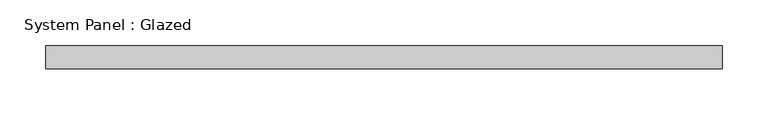
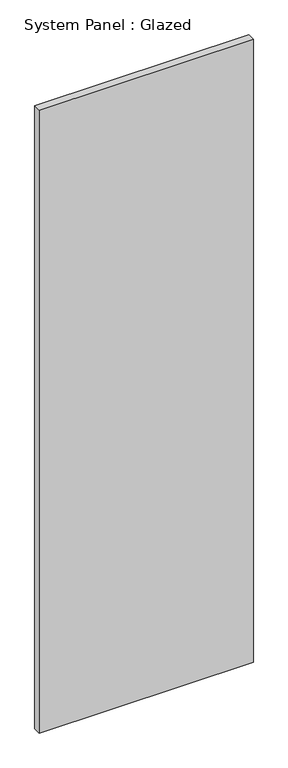
"""IFC4 building model written with IfcOpenShell, lengths in millimetres: plate geometry, System Panel : Glazed."""

from ifc_helpers import new_model, si_unit, origin, origin_with_axes, place, context, project, spatial, polyline, outline, extrude, source, transform, mapped, element, save


def system_panel_glazed_5d718544(model_context):
    return source(origin(), model_context, "Body", "SweptSolid", [
        extrude(outline(polyline([(370.4021, 19.05), (-370.4021, 19.05), (-370.4021, 44.45), (370.4021, 44.45), (370.4021, 19.05)])), origin_with_axes(), (0.0, 0.0, 1.0), 2275.4166667),
    ])


if __name__ == "__main__":
    model = new_model("IFC4")
    model_context = context("Model", 3, world=origin())
    ifc_project = project(units=[si_unit("LENGTHUNIT", "METRE", prefix="MILLI")], contexts=[model_context])
    site = spatial("IfcSite", under=ifc_project)
    building = spatial("IfcBuilding", under=site)
    placement = place(None, origin())
    system_panel_glazed_shape = system_panel_glazed_5d718544(model_context)
    element("IfcPlate", 1, ObjectType="System Panel : Glazed", at=placement, inside=building, context=model_context, shape_type="MappedRepresentation", body=[
        mapped(system_panel_glazed_shape, transform((0.0, 0.0, 0.0), x_axis=(1.0, 0.0, 0.0), y_axis=(0.0, 1.0, 0.0), z_axis=(0.0, 0.0, 1.0))),
    ])
    save(model, "model.ifc")

# Revit data of these elements
# Type "System Panel : Glazed"
#   Construction Type Id = "GSP4R"
#   Analytic Construction = "1/8 in Pilkington single glazing"
#   Visual Light Transmittance = 0.9
#   Solar Heat Gain Coefficient = 0.86
#   Heat Transfer Coefficient (U) = 1.18115 BTU/(h·ft²·°F)
#   Define Thermal Properties by = 1
# Element 1 (IfcPlate, "System Panel : Glazed")
#   Materials on its faces: "Glass"
# Materials
#   "Glass": class "Glass", colour RGB 0 128 192, transparency 0.75, Description = "Soda Lime Glass", Cost = 0
